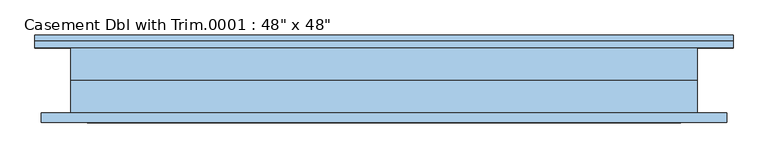
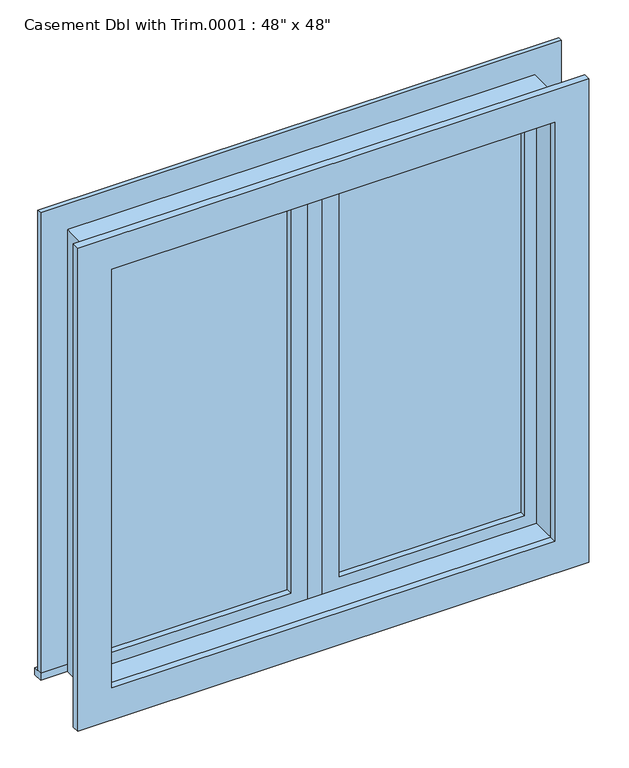
"""IFC4 building model written with IfcOpenShell, lengths in millimetres: window geometry."""

from ifc_helpers import new_model, si_unit, frame, origin, place, context, project, spatial, polyline, outline, extrude, source, transform, mapped, element, save


def window_40d2abec(model_context):
    return source(origin(), model_context, "Body", "SweptSolid", [
        extrude(outline(polyline([(63.5, 47.625), (546.1, 47.625), (546.1, 34.925), (63.5, 34.925), (63.5, 47.625)])), frame((0.0, 0.0, 977.9), z_axis=(0.0, 0.0, 1.0), x_axis=(1.0, 0.0, 0.0)), (0.0, 0.0, 1.0), 1092.2),
        extrude(outline(polyline([(2114.55, 19.05), (933.45, 19.05), (933.45, 590.55), (2114.55, 590.55), (2114.55, 19.05)]), holes=[polyline([(2070.1, 63.5), (2070.1, 546.1), (977.9, 546.1), (977.9, 63.5), (2070.1, 63.5)])]), frame((0.0, 19.05, 0.0), z_axis=(0.0, 1.0, 0.0), x_axis=(0.0, 0.0, 1.0)), (0.0, 0.0, 1.0), 44.45),
        extrude(outline(polyline([(19.05, 19.05), (-19.05, 19.05), (-19.05, 82.55), (19.05, 82.55), (19.05, 19.05)])), frame((0.0, 0.0, 933.45), z_axis=(0.0, 0.0, 1.0), x_axis=(1.0, 0.0, 0.0)), (0.0, 0.0, 1.0), 1181.1),
        extrude(outline(polyline([(-679.45, 107.95), (679.45, 107.95), (679.45, 82.55), (-679.45, 82.55), (-679.45, 107.95)])), frame((0.0, 0.0, 914.4), z_axis=(0.0, 0.0, 1.0), x_axis=(1.0, 0.0, 0.0)), (0.0, 0.0, 1.0), 19.05),
        extrude(outline(polyline([(2114.55, -590.55), (2114.55, 590.55), (933.45, 590.55), (933.45, 679.45), (2203.45, 679.45), (2203.45, -679.45), (933.45, -679.45), (933.45, -590.55), (2114.55, -590.55)])), frame((0.0, 82.55, 0.0), z_axis=(0.0, 1.0, 0.0), x_axis=(0.0, 0.0, 1.0)), (0.0, 0.0, 1.0), 12.7),
        extrude(outline(polyline([(2190.75, 666.75), (2190.75, -666.75), (857.25, -666.75), (857.25, 666.75), (2190.75, 666.75)]), holes=[polyline([(2101.85, 577.85), (946.15, 577.85), (946.15, -577.85), (2101.85, -577.85), (2101.85, 577.85)])]), frame((0.0, -63.5, 0.0), z_axis=(0.0, 1.0, 0.0), x_axis=(0.0, 0.0, 1.0)), (0.0, 0.0, 1.0), 19.05),
        extrude(outline(polyline([(-63.5, 34.925), (-546.1, 34.925), (-546.1, 47.625), (-63.5, 47.625), (-63.5, 34.925)])), frame((0.0, 0.0, 977.9), z_axis=(0.0, 0.0, 1.0), x_axis=(1.0, 0.0, 0.0)), (0.0, 0.0, 1.0), 1092.2),
        extrude(outline(polyline([(2114.55, -590.55), (933.45, -590.55), (933.45, -19.05), (2114.55, -19.05), (2114.55, -590.55)]), holes=[polyline([(2070.1, -546.1), (2070.1, -63.5), (977.9, -63.5), (977.9, -546.1), (2070.1, -546.1)])]), frame((0.0, 19.05, 0.0), z_axis=(0.0, 1.0, 0.0), x_axis=(0.0, 0.0, 1.0)), (0.0, 0.0, 1.0), 44.45),
        extrude(outline(polyline([(2133.6, -609.6), (914.4, -609.6), (914.4, 609.6), (2133.6, 609.6), (2133.6, -609.6)]), holes=[polyline([(2101.85, -577.85), (2101.85, 577.85), (946.15, 577.85), (946.15, -577.85), (2101.85, -577.85)])]), frame((0.0, -44.45, 0.0), z_axis=(0.0, 1.0, 0.0), x_axis=(0.0, 0.0, 1.0)), (0.0, 0.0, 1.0), 63.5),
        extrude(outline(polyline([(2133.6, 609.6), (2133.6, -609.6), (914.4, -609.6), (914.4, 609.6), (2133.6, 609.6)]), holes=[polyline([(2114.55, 590.55), (933.45, 590.55), (933.45, -590.55), (2114.55, -590.55), (2114.55, 590.55)])]), frame((0.0, 19.05, 0.0), z_axis=(0.0, 1.0, 0.0), x_axis=(0.0, 0.0, 1.0)), (0.0, 0.0, 1.0), 63.5),
    ])


if __name__ == "__main__":
    model = new_model("IFC4")
    model_context = context("Model", 3, world=origin())
    ifc_project = project(units=[si_unit("LENGTHUNIT", "METRE", prefix="MILLI")], contexts=[model_context])
    site = spatial("IfcSite", under=ifc_project)
    building = spatial("IfcBuilding", under=site)
    placement = place(None, origin())
    window_shape = window_40d2abec(model_context)
    element("IfcWindow", 1, ObjectType="Casement Dbl with Trim.0001 : 48\" x 48\"", at=placement, inside=building, context=model_context, shape_type="MappedRepresentation", body=[
        mapped(window_shape, transform((0.0, 0.0, 0.0), x_axis=(1.0, 0.0, 0.0), y_axis=(0.0, 1.0, 0.0), z_axis=(0.0, 0.0, 1.0))),
    ])
    save(model, "model.ifc")

# Revit data of these elements
# Type "Casement Dbl with Trim.0001 : 48\" x 48\""
#   Type Mark = "10"
#   Construction Type Id = "GSP4R"
#   Assembly Code = "B2020100"
#   Analytic Construction = "1/8 in Pilkington single glazing"
#   Visual Light Transmittance = 0.9
#   Solar Heat Gain Coefficient = 0.78
#   Heat Transfer Coefficient (U) = 0.6496 BTU/(h·ft²·°F)
#   Height = 4' - 0"
#   Default Sill Height = 3' - 0"
#   Trim Projection - Ext. = 0' - 0 1/2"
#   Trim Projection - Int. = 0' - 0 3/4"
#   Trim Width - Exterior = 0' - 3 1/2"
#   Trim Width - Interior = 0' - 3 1/2"
#   Width = 4' - 0"
#   Window Inset = 0' - 0 3/4"
#   Define Thermal Properties by = 1
#   Glass Pane Material = Glass
#   Sash Material = Sash
#   Trim Exterior Material = Trim
#   Trim Interior Material = Trim
#   Wall Closure = (empty or 0)
# Element 1 (IfcWindow, "Casement Dbl with Trim.0001 : 48\" x 48\"")
#   Materials on its faces: "Sash", "Trim", "Glass"
# Materials
#   "Glass": class "Glass", colour RGB 0 128 192, transparency 0.75, Description = "Soda Lime Glass", Cost = 0
#   "Sash": class "Wood", colour RGB 224 178 126, transparency 0
#   "Trim": class "Wood", colour RGB 224 178 126, transparency 0
